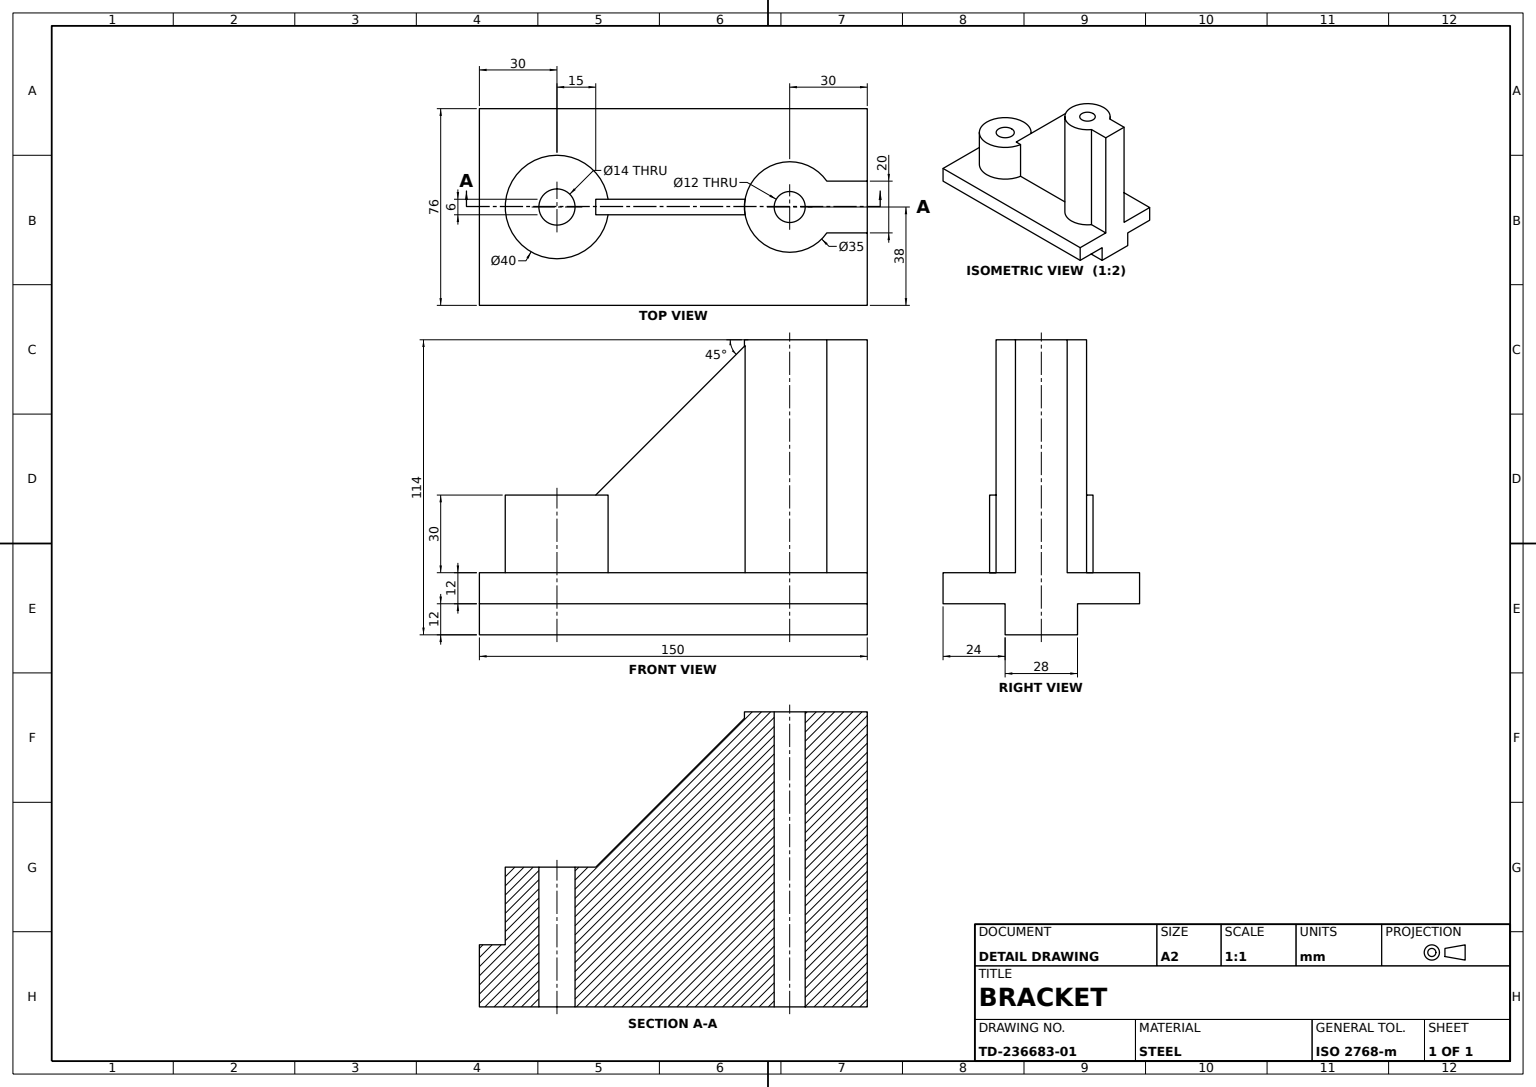
SolidWorks part; units mm, degrees
material "Plain Carbon Steel"
ref_plane "Front Plane" through (0, 0, 0) normal (0, 0, 1) x (1, 0, 0)
ref_plane "Top Plane" through (0, 0, 0) normal (0, 1, 0) x (1, 0, 0)
ref_plane "Right Plane" through (0, 0, 0) normal (1, 0, 0) x (0, 0, -1)
sketch "Base Plate Profile" plane through (0, 0, 0) normal (1, 0, 0) x (0, 0, -1)
  line L0 (0, 0) -> (0, 12)
  line L1 (0, 12) -> (76, 12)
  line L2 (76, 12) -> (76, 0)
  line L3 (76, 0) -> (52, 0)
  line L4 (52, 0) -> (52, -12)
  line L5 (52, -12) -> (24, -12)
  line L6 (24, -12) -> (24, 0)
  line L7 (24, 0) -> (0, 0)
  dimension "D1" = 12
  dimension "D2" = 24
  dimension "D3" = 28
  dimension "D4" = 24
  dimension "D5" = 12
extrude "Base Plate" add sketch "Base Plate Profile" along normal blind 150
ref_plane "Web Rib Plane" through (0, 0, -38) normal (0, 0, 1) x (1, 0, 0)
sketch "Web Rib Profile" plane through (0, 0, -38) normal (0, 0, 1) x (1, 0, 0)
  line L0 (75, 12) -> (105, 12)
  line L1 (150, 12) -> (0, 12) construction
  line L2 (105, 12) -> (105, 102)
  line L3 (105, 102) -> (45, 42)
  line L4 (45, 42) -> (45, 12)
  line L5 (45, 12) -> (75, 12)
  dimension "D1" = 90
  dimension "D2" = 30
  dimension "D3" = 30
  dimension "D4" = 30
extrude "Web Rib" add sketch "Web Rib Profile" along normal mid plane 6
sketch "Tall Boss Profile" plane through (0, 12, 0) normal (0, 1, 0) x (1, 0, 0)
  line L0 (150, 76) -> (150, 0) construction
  line L1 (150, 0) -> (0, 0) construction
  circle A0 centre (120, 38) radius 17.5
  dimension "D1" = 35
  dimension "D2" = 30
  dimension "D3" = 38
extrude "Tall Boss Ø35" add sketch "Tall Boss Profile" along normal blind 90
sketch "Tall Boss Bore Profile" plane through (0, 102, 0) normal (0, 1, 0) x (1, 0, 0)
  circle A0 centre (120, 38) radius 6
  dimension "D1" = 12
extrude "Tall Boss Bore Ø12" cut sketch "Tall Boss Bore Profile" against normal through all
sketch "Short Boss Profile" plane through (0, 12, 0) normal (0, 1, 0) x (1, 0, 0)
  line L0 (150, 0) -> (0, 0) construction
  line L1 (0, 76) -> (0, 0) construction
  circle A0 centre (30, 38) radius 20
  dimension "D1" = 40
  dimension "D2" = 38
  dimension "D3" = 30
extrude "Short Boss Ø40" add sketch "Short Boss Profile" along normal blind 30
sketch "Short Boss Bore Profile" plane through (0, 42, 0) normal (0, 1, 0) x (1, 0, 0)
  circle A0 centre (30, 38) radius 7
  dimension "D1" = 14
extrude "Short Boss Bore Ø14" cut sketch "Short Boss Bore Profile" against normal through all
sketch "Side Lug Profile" plane through (150, 0, 0) normal (1, 0, 0) x (0, 0, -1)
  line L0 (38, 12) -> (28, 12)
  line L1 (76, 12) -> (0, 12) construction
  line L2 (28, 12) -> (28, 102)
  line L3 (55.5, 102) -> (20.5, 102) construction
  line L4 (28, 102) -> (48, 102)
  line L5 (44, 102) -> (32, 102) construction
  line L6 (48, 102) -> (48, 12)
  line L7 (48, 12) -> (38, 12)
  dimension "D1" = 10
  dimension "D2" = 10
extrude "Side Lug" add sketch "Side Lug Profile" against normal blind 20
ref_plane "Plane1" through (0, 0, -38) normal (0, 0, 1) x (1, 0, 0)
